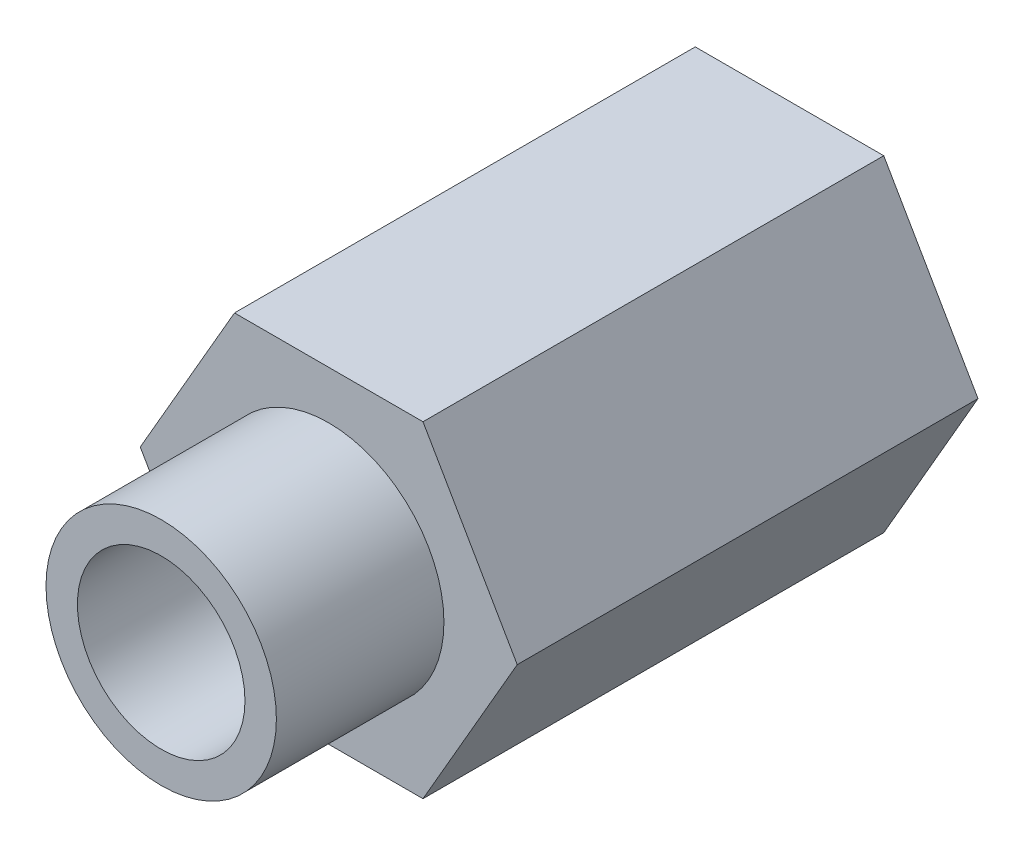
ISO-10303-21;
HEADER;
FILE_DESCRIPTION(('STEP AP214'),'2;1');
FILE_NAME('part.step','',(''),(''),'','','');
FILE_SCHEMA(('AUTOMOTIVE_DESIGN { 1 0 10303 214 1 1 1 1 }'));
ENDSEC;
DATA;
#1=APPLICATION_CONTEXT('core data for automotive mechanical design processes');
#2=APPLICATION_PROTOCOL_DEFINITION('international standard','automotive_design',2000,#1);
#3=PRODUCT_CONTEXT('',#1,'mechanical');
#4=PRODUCT('Part','Part','',(#3));
#5=PRODUCT_RELATED_PRODUCT_CATEGORY('part','',(#4));
#6=PRODUCT_DEFINITION_FORMATION('','',#4);
#7=PRODUCT_DEFINITION_CONTEXT('part definition',#1,'design');
#8=PRODUCT_DEFINITION('design','',#6,#7);
#9=PRODUCT_DEFINITION_SHAPE('','',#8);
#10=(LENGTH_UNIT() NAMED_UNIT(*) SI_UNIT(.MILLI.,.METRE.));
#11=(NAMED_UNIT(*) PLANE_ANGLE_UNIT() SI_UNIT($,.RADIAN.));
#12=(NAMED_UNIT(*) SI_UNIT($,.STERADIAN.) SOLID_ANGLE_UNIT());
#13=UNCERTAINTY_MEASURE_WITH_UNIT(LENGTH_MEASURE(1.E-05),#10,'distance_accuracy_value','');
#14=(GEOMETRIC_REPRESENTATION_CONTEXT(3) GLOBAL_UNCERTAINTY_ASSIGNED_CONTEXT((#13)) GLOBAL_UNIT_ASSIGNED_CONTEXT((#10,
#11,#12)) REPRESENTATION_CONTEXT('',''));
#15=CARTESIAN_POINT('',(0.,0.,0.));
#16=DIRECTION('',(0.,0.,1.));
#17=DIRECTION('',(1.,0.,0.));
#18=AXIS2_PLACEMENT_3D('',#15,#16,#17);
#19=CARTESIAN_POINT('',(0.,0.,0.));
#20=DIRECTION('',(0.,0.,1.));
#21=DIRECTION('',(1.,0.,0.));
#22=AXIS2_PLACEMENT_3D('',#19,#20,#21);
#23=CYLINDRICAL_SURFACE('',#22,4.);
#24=CARTESIAN_POINT('',(0.,0.,30.));
#25=DIRECTION('',(0.,0.,1.));
#26=DIRECTION('',(1.,0.,0.));
#27=AXIS2_PLACEMENT_3D('',#24,#25,#26);
#28=CIRCLE('',#27,4.);
#29=CARTESIAN_POINT('',(4.,0.,30.));
#30=VERTEX_POINT('',#29);
#31=EDGE_CURVE('E157',#30,#30,#28,.T.);
#32=ORIENTED_EDGE('',*,*,#31,.T.);
#33=EDGE_LOOP('',(#32));
#34=FACE_BOUND('',#33,.T.);
#35=CARTESIAN_POINT('',(0.,0.,15.));
#36=DIRECTION('',(0.,0.,-1.));
#37=DIRECTION('',(-1.,0.,0.));
#38=AXIS2_PLACEMENT_3D('',#35,#36,#37);
#39=CIRCLE('',#38,4.);
#40=CARTESIAN_POINT('',(-4.,0.,15.));
#41=VERTEX_POINT('',#40);
#42=EDGE_CURVE('E43',#41,#41,#39,.F.);
#43=ORIENTED_EDGE('',*,*,#42,.F.);
#44=EDGE_LOOP('',(#43));
#45=FACE_BOUND('',#44,.T.);
#46=ADVANCED_FACE('F39',(#34,#45),#23,.F.);
#47=CARTESIAN_POINT('',(4.50000000000008,-7.79422863405988,22.));
#48=DIRECTION('',(-0.866025403784441,0.499999999999995,0.));
#49=DIRECTION('',(-0.499999999999995,-0.866025403784441,0.));
#50=AXIS2_PLACEMENT_3D('',#47,#48,#49);
#51=PLANE('',#50);
#52=DIRECTION('',(0.499999999999995,0.866025403784441,0.));
#53=VECTOR('',#52,1.);
#54=CARTESIAN_POINT('',(4.50000000000008,-7.79422863405988,0.));
#55=LINE('',#54,#53);
#56=CARTESIAN_POINT('',(4.50000000000008,-7.79422863405988,0.));
#57=VERTEX_POINT('',#56);
#58=CARTESIAN_POINT('',(8.99999999999998,0.,0.));
#59=VERTEX_POINT('',#58);
#60=EDGE_CURVE('E130',#57,#59,#55,.T.);
#61=ORIENTED_EDGE('',*,*,#60,.T.);
#62=DIRECTION('',(0.,0.,-1.));
#63=VECTOR('',#62,1.);
#64=CARTESIAN_POINT('',(8.99999999999998,0.,22.));
#65=LINE('',#64,#63);
#66=CARTESIAN_POINT('',(8.99999999999998,0.,22.));
#67=VERTEX_POINT('',#66);
#68=EDGE_CURVE('E47',#67,#59,#65,.T.);
#69=ORIENTED_EDGE('',*,*,#68,.F.);
#70=DIRECTION('',(0.499999999999995,0.866025403784441,0.));
#71=VECTOR('',#70,1.);
#72=CARTESIAN_POINT('',(4.50000000000008,-7.79422863405988,22.));
#73=LINE('',#72,#71);
#74=CARTESIAN_POINT('',(4.50000000000008,-7.79422863405988,22.));
#75=VERTEX_POINT('',#74);
#76=EDGE_CURVE('E140',#75,#67,#73,.T.);
#77=ORIENTED_EDGE('',*,*,#76,.F.);
#78=DIRECTION('',(0.,0.,-1.));
#79=VECTOR('',#78,1.);
#80=CARTESIAN_POINT('',(4.50000000000008,-7.79422863405988,22.));
#81=LINE('',#80,#79);
#82=EDGE_CURVE('E125',#75,#57,#81,.T.);
#83=ORIENTED_EDGE('',*,*,#82,.T.);
#84=EDGE_LOOP('',(#61,#69,#77,#83));
#85=FACE_BOUND('',#84,.T.);
#86=ADVANCED_FACE('F41',(#85),#51,.F.);
#87=CARTESIAN_POINT('',(8.99999999999998,0.,22.));
#88=DIRECTION('',(-0.866025403784438,-0.500000000000001,0.));
#89=DIRECTION('',(0.500000000000001,-0.866025403784438,0.));
#90=AXIS2_PLACEMENT_3D('',#87,#88,#89);
#91=PLANE('',#90);
#92=DIRECTION('',(-0.500000000000001,0.866025403784438,0.));
#93=VECTOR('',#92,1.);
#94=CARTESIAN_POINT('',(8.99999999999998,0.,0.));
#95=LINE('',#94,#93);
#96=CARTESIAN_POINT('',(4.49999999999997,7.79422863405994,0.));
#97=VERTEX_POINT('',#96);
#98=EDGE_CURVE('E128',#59,#97,#95,.T.);
#99=ORIENTED_EDGE('',*,*,#98,.T.);
#100=DIRECTION('',(0.,0.,-1.));
#101=VECTOR('',#100,1.);
#102=CARTESIAN_POINT('',(4.49999999999997,7.79422863405994,22.));
#103=LINE('',#102,#101);
#104=CARTESIAN_POINT('',(4.49999999999997,7.79422863405994,22.));
#105=VERTEX_POINT('',#104);
#106=EDGE_CURVE('E142',#105,#97,#103,.T.);
#107=ORIENTED_EDGE('',*,*,#106,.F.);
#108=DIRECTION('',(-0.500000000000001,0.866025403784438,0.));
#109=VECTOR('',#108,1.);
#110=CARTESIAN_POINT('',(8.99999999999998,0.,22.));
#111=LINE('',#110,#109);
#112=EDGE_CURVE('E96',#67,#105,#111,.T.);
#113=ORIENTED_EDGE('',*,*,#112,.F.);
#114=ORIENTED_EDGE('',*,*,#68,.T.);
#115=EDGE_LOOP('',(#99,#107,#113,#114));
#116=FACE_BOUND('',#115,.T.);
#117=ADVANCED_FACE('F144',(#116),#91,.F.);
#118=CARTESIAN_POINT('',(4.49999999999997,7.79422863405994,22.));
#119=DIRECTION('',(0.,-1.,0.));
#120=DIRECTION('',(1.,0.,0.));
#121=AXIS2_PLACEMENT_3D('',#118,#119,#120);
#122=PLANE('',#121);
#123=DIRECTION('',(-1.,0.,0.));
#124=VECTOR('',#123,1.);
#125=CARTESIAN_POINT('',(4.49999999999997,7.79422863405994,0.));
#126=LINE('',#125,#124);
#127=CARTESIAN_POINT('',(-4.50000000000002,7.79422863405991,0.));
#128=VERTEX_POINT('',#127);
#129=EDGE_CURVE('E134',#97,#128,#126,.T.);
#130=ORIENTED_EDGE('',*,*,#129,.T.);
#131=DIRECTION('',(0.,0.,-1.));
#132=VECTOR('',#131,1.);
#133=CARTESIAN_POINT('',(-4.50000000000002,7.79422863405991,22.));
#134=LINE('',#133,#132);
#135=CARTESIAN_POINT('',(-4.50000000000002,7.79422863405991,22.));
#136=VERTEX_POINT('',#135);
#137=EDGE_CURVE('E119',#136,#128,#134,.T.);
#138=ORIENTED_EDGE('',*,*,#137,.F.);
#139=DIRECTION('',(-1.,0.,0.));
#140=VECTOR('',#139,1.);
#141=CARTESIAN_POINT('',(4.49999999999997,7.79422863405994,22.));
#142=LINE('',#141,#140);
#143=EDGE_CURVE('E108',#105,#136,#142,.T.);
#144=ORIENTED_EDGE('',*,*,#143,.F.);
#145=ORIENTED_EDGE('',*,*,#106,.T.);
#146=EDGE_LOOP('',(#130,#138,#144,#145));
#147=FACE_BOUND('',#146,.T.);
#148=ADVANCED_FACE('F153',(#147),#122,.F.);
#149=CARTESIAN_POINT('',(-4.50000000000002,7.79422863405991,22.));
#150=DIRECTION('',(0.866025403784442,-0.499999999999995,0.));
#151=DIRECTION('',(0.499999999999995,0.866025403784442,0.));
#152=AXIS2_PLACEMENT_3D('',#149,#150,#151);
#153=PLANE('',#152);
#154=DIRECTION('',(-0.499999999999995,-0.866025403784441,0.));
#155=VECTOR('',#154,1.);
#156=CARTESIAN_POINT('',(-4.50000000000002,7.79422863405991,0.));
#157=LINE('',#156,#155);
#158=CARTESIAN_POINT('',(-8.99999999999998,0.,0.));
#159=VERTEX_POINT('',#158);
#160=EDGE_CURVE('E117',#128,#159,#157,.T.);
#161=ORIENTED_EDGE('',*,*,#160,.T.);
#162=DIRECTION('',(0.,0.,-1.));
#163=VECTOR('',#162,1.);
#164=CARTESIAN_POINT('',(-8.99999999999998,0.,22.));
#165=LINE('',#164,#163);
#166=CARTESIAN_POINT('',(-8.99999999999998,0.,22.));
#167=VERTEX_POINT('',#166);
#168=EDGE_CURVE('E111',#167,#159,#165,.T.);
#169=ORIENTED_EDGE('',*,*,#168,.F.);
#170=DIRECTION('',(-0.499999999999995,-0.866025403784441,0.));
#171=VECTOR('',#170,1.);
#172=CARTESIAN_POINT('',(-4.50000000000002,7.79422863405991,22.));
#173=LINE('',#172,#171);
#174=EDGE_CURVE('E103',#136,#167,#173,.T.);
#175=ORIENTED_EDGE('',*,*,#174,.F.);
#176=ORIENTED_EDGE('',*,*,#137,.T.);
#177=EDGE_LOOP('',(#161,#169,#175,#176));
#178=FACE_BOUND('',#177,.T.);
#179=ADVANCED_FACE('F113',(#178),#153,.F.);
#180=CARTESIAN_POINT('',(-8.99999999999998,0.,22.));
#181=DIRECTION('',(0.866025403784435,0.500000000000007,0.));
#182=DIRECTION('',(-0.500000000000007,0.866025403784434,0.));
#183=AXIS2_PLACEMENT_3D('',#180,#181,#182);
#184=PLANE('',#183);
#185=DIRECTION('',(0.500000000000007,-0.866025403784435,0.));
#186=VECTOR('',#185,1.);
#187=CARTESIAN_POINT('',(-8.99999999999998,0.,0.));
#188=LINE('',#187,#186);
#189=CARTESIAN_POINT('',(-4.49999999999992,-7.79422863405997,0.));
#190=VERTEX_POINT('',#189);
#191=EDGE_CURVE('E82',#159,#190,#188,.T.);
#192=ORIENTED_EDGE('',*,*,#191,.T.);
#193=DIRECTION('',(0.,0.,-1.));
#194=VECTOR('',#193,1.);
#195=CARTESIAN_POINT('',(-4.49999999999992,-7.79422863405997,22.));
#196=LINE('',#195,#194);
#197=CARTESIAN_POINT('',(-4.49999999999992,-7.79422863405997,22.));
#198=VERTEX_POINT('',#197);
#199=EDGE_CURVE('E118',#198,#190,#196,.T.);
#200=ORIENTED_EDGE('',*,*,#199,.F.);
#201=DIRECTION('',(0.500000000000007,-0.866025403784435,0.));
#202=VECTOR('',#201,1.);
#203=CARTESIAN_POINT('',(-8.99999999999998,0.,22.));
#204=LINE('',#203,#202);
#205=EDGE_CURVE('E110',#167,#198,#204,.T.);
#206=ORIENTED_EDGE('',*,*,#205,.F.);
#207=ORIENTED_EDGE('',*,*,#168,.T.);
#208=EDGE_LOOP('',(#192,#200,#206,#207));
#209=FACE_BOUND('',#208,.T.);
#210=ADVANCED_FACE('F122',(#209),#184,.F.);
#211=CARTESIAN_POINT('',(-4.49999999999992,-7.79422863405997,22.));
#212=DIRECTION('',(0.,1.,0.));
#213=DIRECTION('',(-1.,0.,0.));
#214=AXIS2_PLACEMENT_3D('',#211,#212,#213);
#215=PLANE('',#214);
#216=DIRECTION('',(1.,0.,0.));
#217=VECTOR('',#216,1.);
#218=CARTESIAN_POINT('',(-4.49999999999992,-7.79422863405997,0.));
#219=LINE('',#218,#217);
#220=EDGE_CURVE('E87',#190,#57,#219,.T.);
#221=ORIENTED_EDGE('',*,*,#220,.T.);
#222=ORIENTED_EDGE('',*,*,#82,.F.);
#223=DIRECTION('',(1.,0.,0.));
#224=VECTOR('',#223,1.);
#225=CARTESIAN_POINT('',(-4.49999999999992,-7.79422863405997,22.));
#226=LINE('',#225,#224);
#227=EDGE_CURVE('E59',#198,#75,#226,.T.);
#228=ORIENTED_EDGE('',*,*,#227,.F.);
#229=ORIENTED_EDGE('',*,*,#199,.T.);
#230=EDGE_LOOP('',(#221,#222,#228,#229));
#231=FACE_BOUND('',#230,.T.);
#232=ADVANCED_FACE('F193',(#231),#215,.F.);
#233=CARTESIAN_POINT('',(0.,0.,22.));
#234=DIRECTION('',(0.,0.,1.));
#235=DIRECTION('',(1.,0.,0.));
#236=AXIS2_PLACEMENT_3D('',#233,#234,#235);
#237=PLANE('',#236);
#238=CARTESIAN_POINT('',(0.,0.,22.));
#239=DIRECTION('',(0.,0.,1.));
#240=DIRECTION('',(1.,0.,0.));
#241=AXIS2_PLACEMENT_3D('',#238,#239,#240);
#242=CIRCLE('',#241,5.5);
#243=CARTESIAN_POINT('',(5.5,0.,22.));
#244=VERTEX_POINT('',#243);
#245=EDGE_CURVE('E11',#244,#244,#242,.T.);
#246=ORIENTED_EDGE('',*,*,#245,.F.);
#247=EDGE_LOOP('',(#246));
#248=FACE_BOUND('',#247,.T.);
#249=ORIENTED_EDGE('',*,*,#76,.T.);
#250=ORIENTED_EDGE('',*,*,#112,.T.);
#251=ORIENTED_EDGE('',*,*,#143,.T.);
#252=ORIENTED_EDGE('',*,*,#174,.T.);
#253=ORIENTED_EDGE('',*,*,#205,.T.);
#254=ORIENTED_EDGE('',*,*,#227,.T.);
#255=EDGE_LOOP('',(#249,#250,#251,#252,#253,#254));
#256=FACE_BOUND('',#255,.T.);
#257=ADVANCED_FACE('F104',(#248,#256),#237,.T.);
#258=CARTESIAN_POINT('',(0.,0.,0.));
#259=DIRECTION('',(0.,0.,1.));
#260=DIRECTION('',(1.,0.,0.));
#261=AXIS2_PLACEMENT_3D('',#258,#259,#260);
#262=PLANE('',#261);
#263=CARTESIAN_POINT('',(0.,0.,0.));
#264=DIRECTION('',(0.,0.,-1.));
#265=DIRECTION('',(-1.,0.,0.));
#266=AXIS2_PLACEMENT_3D('',#263,#264,#265);
#267=CIRCLE('',#266,6.);
#268=CARTESIAN_POINT('',(-6.,0.,0.));
#269=VERTEX_POINT('',#268);
#270=EDGE_CURVE('E165',#269,#269,#267,.T.);
#271=ORIENTED_EDGE('',*,*,#270,.F.);
#272=EDGE_LOOP('',(#271));
#273=FACE_BOUND('',#272,.T.);
#274=ORIENTED_EDGE('',*,*,#60,.F.);
#275=ORIENTED_EDGE('',*,*,#220,.F.);
#276=ORIENTED_EDGE('',*,*,#191,.F.);
#277=ORIENTED_EDGE('',*,*,#160,.F.);
#278=ORIENTED_EDGE('',*,*,#129,.F.);
#279=ORIENTED_EDGE('',*,*,#98,.F.);
#280=EDGE_LOOP('',(#274,#275,#276,#277,#278,#279));
#281=FACE_BOUND('',#280,.T.);
#282=ADVANCED_FACE('F147',(#273,#281),#262,.F.);
#283=CARTESIAN_POINT('',(0.,0.,30.));
#284=DIRECTION('',(0.,0.,-1.));
#285=DIRECTION('',(-1.,0.,0.));
#286=AXIS2_PLACEMENT_3D('',#283,#284,#285);
#287=CYLINDRICAL_SURFACE('',#286,5.5);
#288=CARTESIAN_POINT('',(0.,0.,30.));
#289=DIRECTION('',(0.,0.,1.));
#290=DIRECTION('',(1.,0.,0.));
#291=AXIS2_PLACEMENT_3D('',#288,#289,#290);
#292=CIRCLE('',#291,5.5);
#293=CARTESIAN_POINT('',(5.5,0.,30.));
#294=VERTEX_POINT('',#293);
#295=EDGE_CURVE('E131',#294,#294,#292,.T.);
#296=ORIENTED_EDGE('',*,*,#295,.F.);
#297=EDGE_LOOP('',(#296));
#298=FACE_BOUND('',#297,.T.);
#299=ORIENTED_EDGE('',*,*,#245,.T.);
#300=EDGE_LOOP('',(#299));
#301=FACE_BOUND('',#300,.T.);
#302=ADVANCED_FACE('F189',(#298,#301),#287,.T.);
#303=CARTESIAN_POINT('',(0.,0.,30.));
#304=DIRECTION('',(0.,0.,1.));
#305=DIRECTION('',(1.,0.,0.));
#306=AXIS2_PLACEMENT_3D('',#303,#304,#305);
#307=PLANE('',#306);
#308=ORIENTED_EDGE('',*,*,#31,.F.);
#309=EDGE_LOOP('',(#308));
#310=FACE_BOUND('',#309,.T.);
#311=ORIENTED_EDGE('',*,*,#295,.T.);
#312=EDGE_LOOP('',(#311));
#313=FACE_BOUND('',#312,.T.);
#314=ADVANCED_FACE('F186',(#310,#313),#307,.T.);
#315=CARTESIAN_POINT('',(0.,0.,15.));
#316=DIRECTION('',(0.,0.,-1.));
#317=DIRECTION('',(-1.,0.,0.));
#318=AXIS2_PLACEMENT_3D('',#315,#316,#317);
#319=PLANE('',#318);
#320=CARTESIAN_POINT('',(0.,0.,15.));
#321=DIRECTION('',(0.,0.,-1.));
#322=DIRECTION('',(-1.,0.,0.));
#323=AXIS2_PLACEMENT_3D('',#320,#321,#322);
#324=CIRCLE('',#323,6.);
#325=CARTESIAN_POINT('',(-6.,0.,15.));
#326=VERTEX_POINT('',#325);
#327=EDGE_CURVE('E164',#326,#326,#324,.T.);
#328=ORIENTED_EDGE('',*,*,#327,.T.);
#329=EDGE_LOOP('',(#328));
#330=FACE_BOUND('',#329,.T.);
#331=ORIENTED_EDGE('',*,*,#42,.T.);
#332=EDGE_LOOP('',(#331));
#333=FACE_BOUND('',#332,.T.);
#334=ADVANCED_FACE('F172',(#330,#333),#319,.T.);
#335=CARTESIAN_POINT('',(0.,0.,15.));
#336=DIRECTION('',(0.,0.,-1.));
#337=DIRECTION('',(-1.,0.,0.));
#338=AXIS2_PLACEMENT_3D('',#335,#336,#337);
#339=CYLINDRICAL_SURFACE('',#338,6.);
#340=ORIENTED_EDGE('',*,*,#327,.F.);
#341=EDGE_LOOP('',(#340));
#342=FACE_BOUND('',#341,.T.);
#343=ORIENTED_EDGE('',*,*,#270,.T.);
#344=EDGE_LOOP('',(#343));
#345=FACE_BOUND('',#344,.T.);
#346=ADVANCED_FACE('F184',(#342,#345),#339,.F.);
#347=CLOSED_SHELL('',(#46,#86,#117,#148,#179,#210,#232,#257,#282,#302,#314,#334,#346));
#348=MANIFOLD_SOLID_BREP('B2',#347);
#349=ADVANCED_BREP_SHAPE_REPRESENTATION('',(#18,#348),#14);
#350=SHAPE_DEFINITION_REPRESENTATION(#9,#349);
ENDSEC;
END-ISO-10303-21;
